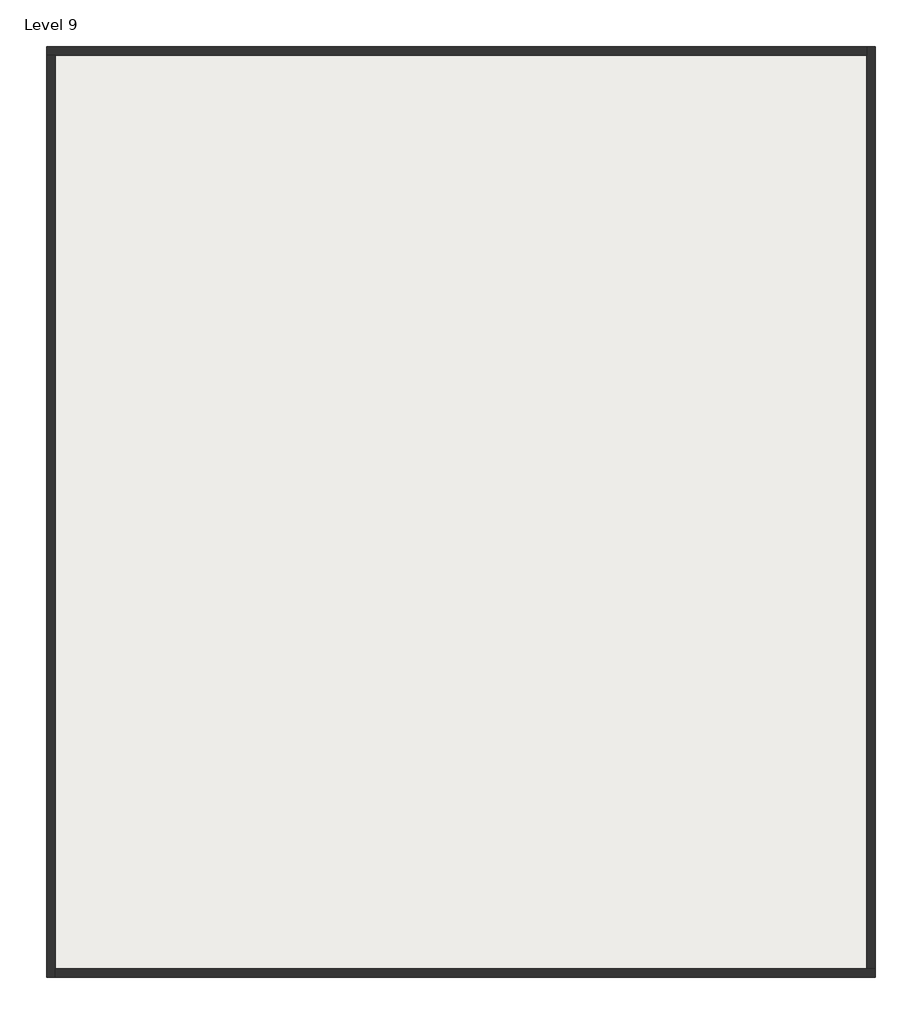
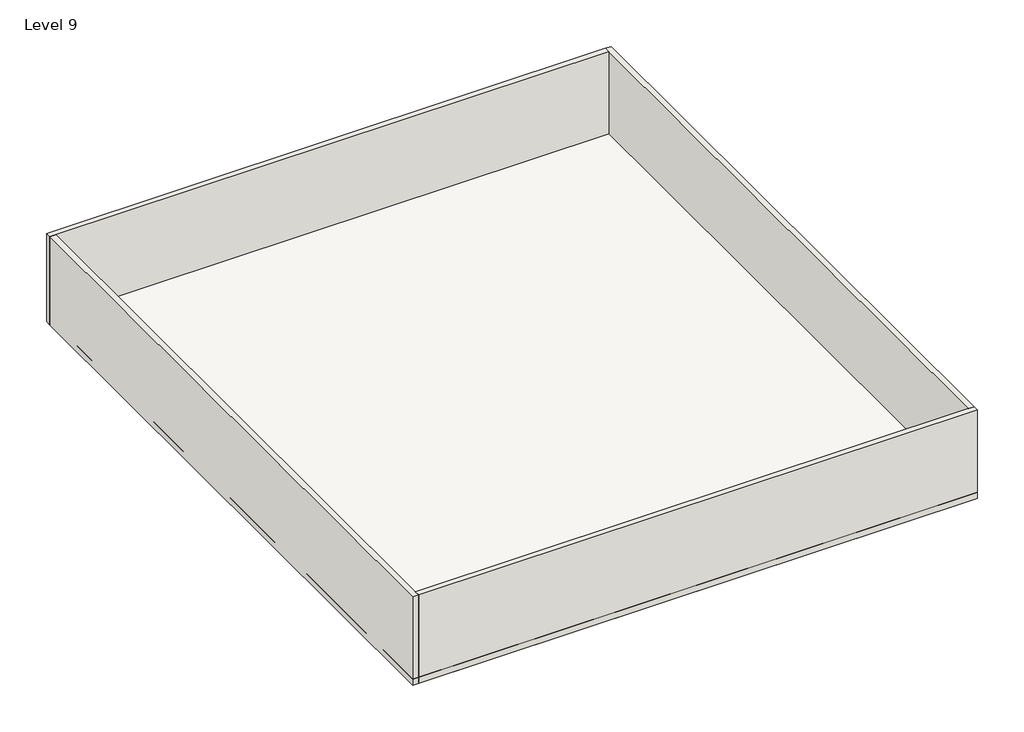
# One storey: 4 walls, 1 roof.
"""IFC4 building model written with IfcOpenShell, lengths in millimetres."""

from ifc_helpers import new_model, si_unit, frame, origin, place, context, project, spatial, polyline, outline, extrude, faceted_brep, element, save

model = new_model("IFC4")

# Units and contexts
model_context = context("Model", 3, world=origin())
ifc_project = project(units=[si_unit("LENGTHUNIT", "METRE", prefix="MILLI")], contexts=[model_context])

# Site, building, storey
site = spatial("IfcSite", under=ifc_project)
building = spatial("IfcBuilding", under=site)
storey = spatial("IfcBuildingStorey", under=building, Name="Level 9", Elevation=9601.2)

# Roof
placement = place(None, origin())
element("IfcRoof", 1, ObjectType="Generic - 9\"", at=placement, inside=storey, context=model_context, shape_type="SweptSolid", body=[
    extrude(outline(polyline([(-10060.7625896, 13609.2178947), (9751.2374104, 13609.2178947), (9751.2374104, -8641.1821053), (-10060.7625896, -8641.1821053), (-10060.7625896, 13609.2178947)])), frame((0.0, 0.0, 9601.2), z_axis=(0.0, 0.0, 1.0), x_axis=(1.0, 0.0, 0.0)), (0.0, 0.0, 1.0), 228.6),
])

# Walls
element("IfcWall", 2, ObjectType="Generic - 8\"", at=placement, inside=storey, context=model_context, shape_type="Brep", body=[
    faceted_brep([(-10060.7625896, 13406.0178947, 9601.2), (-9857.5625896, 13406.0178947, 9601.2), (9548.0374104, 13406.0178947, 9601.2), (9548.0374104, 13406.0178947, 12877.8), (-9857.5625896, 13406.0178947, 12877.8), (-10060.7625896, 13406.0178947, 12877.8), (-10060.7625896, 13609.2178947, 9601.2), (-10060.7625896, 13609.2178947, 12877.8), (9548.0374104, 13609.2178947, 12877.8), (9548.0374104, 13609.2178947, 9601.2)], [[[0, 1, 2, 3, 4, 5]], [[6, 7, 8, 9]], [[2, 1, 0, 6, 9]], [[5, 4, 3, 8, 7]], [[0, 5, 7, 6]], [[3, 2, 9, 8]]]),
])
element("IfcWall", 3, ObjectType="Generic - 8\"", at=placement, inside=storey, context=model_context, shape_type="Brep", body=[
    faceted_brep([(-9857.5625896, -8641.1821053, 9601.2), (-9857.5625896, -8437.9821053, 9601.2), (-9857.5625896, 13406.0178947, 9601.2), (-9857.5625896, 13406.0178947, 12877.8), (-9857.5625896, -8437.9821053, 12877.8), (-9857.5625896, -8641.1821053, 12877.8), (-10060.7625896, -8641.1821053, 9601.2), (-10060.7625896, -8641.1821053, 12877.8), (-10060.7625896, 13406.0178947, 12877.8), (-10060.7625896, 13406.0178947, 9601.2)], [[[0, 1, 2, 3, 4, 5]], [[6, 7, 8, 9]], [[2, 1, 0, 6, 9]], [[5, 4, 3, 8, 7]], [[0, 5, 7, 6]], [[3, 2, 9, 8]]]),
])
element("IfcWall", 4, ObjectType="Generic - 8\"", at=placement, inside=storey, context=model_context, shape_type="Brep", body=[
    faceted_brep([(9751.2374104, -8437.9821053, 9601.2), (9548.0374104, -8437.9821053, 9601.2), (-9857.5625896, -8437.9821053, 9601.2), (-9857.5625896, -8437.9821053, 12877.8), (9548.0374104, -8437.9821053, 12877.8), (9751.2374104, -8437.9821053, 12877.8), (9751.2374104, -8641.1821053, 9601.2), (9751.2374104, -8641.1821053, 12877.8), (-9857.5625896, -8641.1821053, 12877.8), (-9857.5625896, -8641.1821053, 9601.2)], [[[0, 1, 2, 3, 4, 5]], [[6, 7, 8, 9]], [[2, 1, 0, 6, 9]], [[5, 4, 3, 8, 7]], [[0, 5, 7, 6]], [[3, 2, 9, 8]]]),
])
element("IfcWall", 5, ObjectType="Generic - 8\"", at=placement, inside=storey, context=model_context, shape_type="Brep", body=[
    faceted_brep([(9548.0374104, 13609.2178947, 9601.2), (9548.0374104, 13406.0178947, 9601.2), (9548.0374104, -8437.9821053, 9601.2), (9548.0374104, -8437.9821053, 12877.8), (9548.0374104, 13406.0178947, 12877.8), (9548.0374104, 13609.2178947, 12877.8), (9751.2374104, 13609.2178947, 9601.2), (9751.2374104, 13609.2178947, 12877.8), (9751.2374104, -8437.9821053, 12877.8), (9751.2374104, -8437.9821053, 9601.2)], [[[0, 1, 2, 3, 4, 5]], [[6, 7, 8, 9]], [[2, 1, 0, 6, 9]], [[5, 4, 3, 8, 7]], [[0, 5, 7, 6]], [[3, 2, 9, 8]]]),
])

save(model, "model.ifc")

# Revit data of these elements
# Type "Generic - 9\""
#   Assembly Code = "B1020"
#   Layers, outside or top first: 0' - 9" no material (function 1)
# Type "Generic - 8\""
#   Assembly Code = "B2010"
#   Layers, outside or top first: 0' - 8" no material (function 1)
# Element 1 (IfcRoof, "Generic - 9\"")
#   built-in parameter 1001705 = 32.25 (stored number, unit not read)
#   built-in parameter 1001710 = 33615
#   Phase Created = New Construction
#   Materials on its faces: "Default Roof"
# Elements 2, 3, 4, 5 (IfcWall, "Generic - 8\"")
#   Top Offset = 0' - 0"
#   Base Offset = 0' - 0"
#   Unconnected Height = 10' - 9"
#   wall height = 10' - 9"
#   Phase Created = New Construction
#   Base Constraint = Level 9
#   Materials on its faces: "Default Wall"
# Materials
#   "Default Roof": colour RGB 88 101 114, transparency 0
#   "Default Wall": colour RGB 128 128 128, transparency 0
